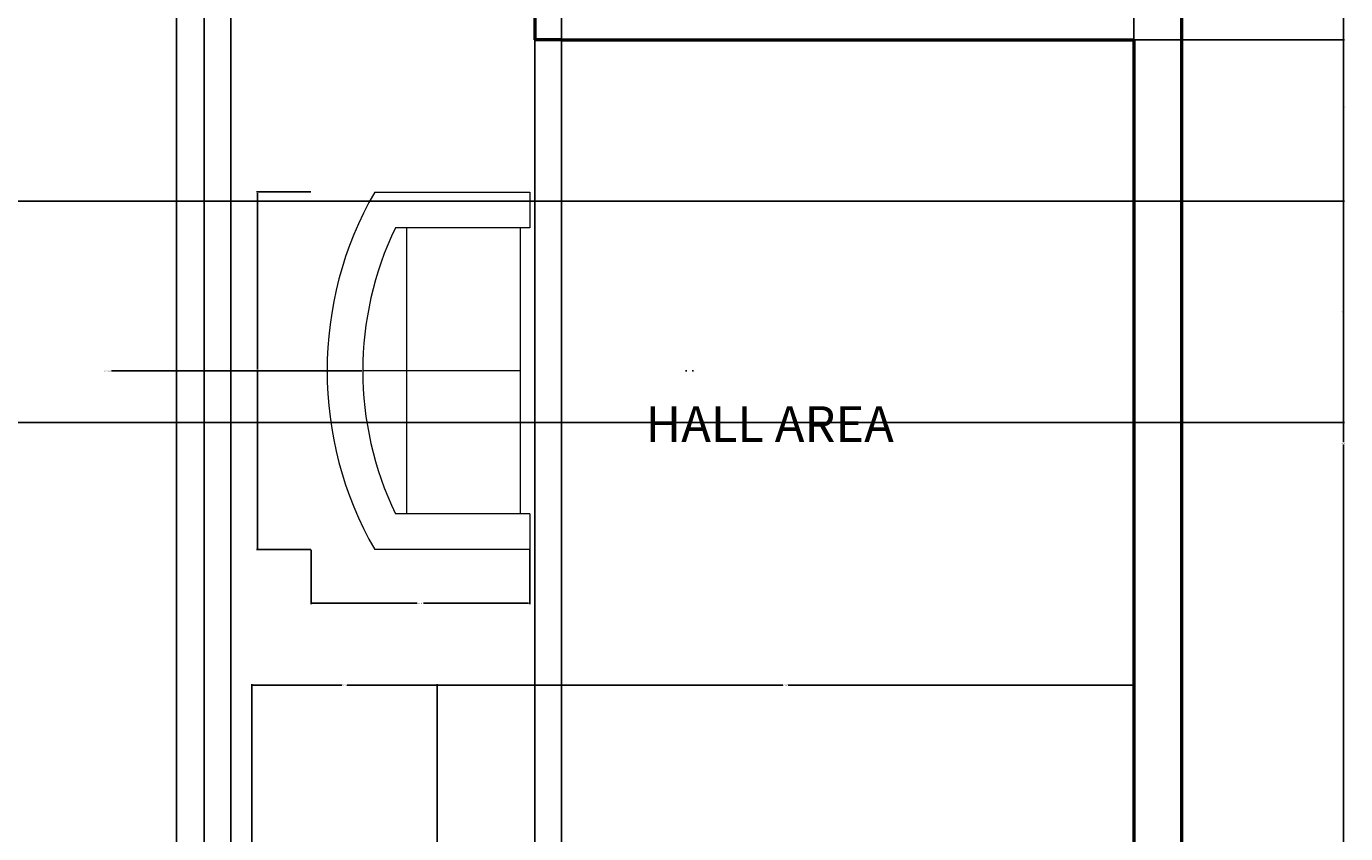
# Model space of a CAD drawing. Units: inches. Extents: x 2907 to 3328, y 1715 to 2286.
# Tile 4 of 5: x 3107 to 3328, y 1969 to 2105. Entities that reach past the tile are written whole.
import ezdxf

# ---------------------------------------------------------------- set-up
doc = ezdxf.new("R2010")
doc.units = ezdxf.units.IN
for name, color, linetype, lineweight in [('A-ANNO-DIMS', 2, 'Continuous', 18), ('A-AREA-IDEN', 7, 'Continuous', 25), ('A-FURN', 8, 'Continuous', 18), ('A-WALL', 7, 'Continuous', 50)]:
    doc.layers.add(name, color=color, linetype=linetype, lineweight=lineweight)
doc.styles.get("Standard").update_dxf_attribs({"font": 'arial.ttf'})
doc.dimstyles.get("Standard").update_dxf_attribs({"dimtxt": 0.18, "dimasz": 0.18, "dimexe": 0.18, "dimexo": 0.0625, "dimgap": 0.09, "dimtad": 0, "dimtih": 1, "dimtoh": 1, "dimdec": 4, "dimzin": 0, "dimdsep": 46, "dimtxsty": 'Standard', "dimcen": 0.09, "dimadec": 0, "dimazin": 0, "dimtfac": 1, "dimtdec": 4, "dimtofl": 0, "dimtmove": 0, "dimatfit": 3, "dimfxl": 1, "dimtolj": 1, "dimtzin": 0, "dimarcsym": 0})

# ---------------------------------------------------------------- blocks, each defined once
blk = doc.blocks.new('Sofa - Roundback Loveseat 5 ft.')
for p, q in [((0, -32.44198), (0, -5.99998)), ((-24, -33.99998), (-24, -11.46958)), ((24.00004, -33.99998), (24.00004, -11.46958)), ((-23.9998, -13.38178), (23.99986, -13.38178)), ((-24, -32.44198), (24.00004, -32.44198))]:
    blk.add_line(p, q)
for points in [[(-24, -33.99998), (-30, -33.99998), (-30, -7.99998)], [(30.00004, -7.99998), (30.00004, -33.99998), (24.00004, -33.99998)]]:
    blk.add_lwpolyline(points)
for centre, radius, start, end in [((0, -60.24998), 60.24998, 60.13715, 119.8628), ((0, -61.38438), 55.38444, 64.32083, 115.6792)]:
    blk.add_arc(centre, radius, start, end)
blk = doc.blocks.new('*D7')
at = {"layer": 'A-ANNO-DIMS', "color": 0, "lineweight": -2, "transparency": 16777216}
for p, q in [((3154.5, 2076.78), (3145.38, 2076.78)), ((3145.56, 2076.6), (3145.56, 2046.96)), ((3145.56, 2016.96), (3145.56, 2046.59)), ((3154.5, 2016.78), (3145.38, 2016.78))]:
    blk.add_line(p, q, dxfattribs=at)
at = {"layer": 'A-ANNO-DIMS', "color": 0, "transparency": 16777216}
for points in [[(3145.53, 2076.6), (3145.59, 2076.6), (3145.56, 2076.78)], [(3145.53, 2016.96), (3145.59, 2016.96), (3145.56, 2016.78)]]:
    blk.add_solid(points, dxfattribs=at)
at = {"layer": 'Defpoints', "color": 0, "transparency": 16777216}
for p in [(3145.56, 2076.78), (3154.56, 2076.78), (3154.56, 2016.78)]:
    blk.add_point(p, dxfattribs=at)
at = {"layer": 'A-ANNO-DIMS', "color": 0, "transparency": 16777216, "insert": (3145.56, 2046.78), "char_height": 0.18, "attachment_point": 5}
blk.add_mtext('\\A1;LOVESEAT 60 TYP.', dxfattribs=at)
blk = doc.blocks.new('*D8')
at = {"layer": 'A-ANNO-DIMS', "color": 0, "lineweight": -2, "transparency": 16777216}
for p, q in [((3154.56, 2016.72), (3154.56, 2007.6)), ((3191.23, 2016.72), (3191.23, 2007.6)), ((3154.74, 2007.78), (3172.37, 2007.78)), ((3191.05, 2007.78), (3173.42, 2007.78))]:
    blk.add_line(p, q, dxfattribs=at)
at = {"layer": 'A-ANNO-DIMS', "color": 0, "transparency": 16777216}
for points in [[(3154.74, 2007.81), (3154.74, 2007.75), (3154.56, 2007.78)], [(3191.05, 2007.81), (3191.05, 2007.75), (3191.23, 2007.78)]]:
    blk.add_solid(points, dxfattribs=at)
at = {"layer": 'Defpoints', "color": 0, "transparency": 16777216}
for p in [(3154.56, 2016.78), (3191.23, 2016.78), (3154.56, 2007.78)]:
    blk.add_point(p, dxfattribs=at)
at = {"layer": 'A-ANNO-DIMS', "color": 0, "transparency": 16777216, "insert": (3172.9, 2007.78), "char_height": 0.18, "attachment_point": 5}
blk.add_mtext('\\A1;37 TYP.', dxfattribs=at)
blk = doc.blocks.new('*D17')
at = {"layer": 'A-ANNO-DIMS', "color": 0, "lineweight": -2, "transparency": 16777216}
for p, q in [((3080.59, 2250.77), (3080.59, 1715.5)), ((3192.09, 2250.77), (3192.09, 1715.5)), ((3080.77, 1715.68), (3135.95, 1715.68)), ((3191.91, 1715.68), (3136.73, 1715.68))]:
    blk.add_line(p, q, dxfattribs=at)
at = {"layer": 'A-ANNO-DIMS', "color": 0, "transparency": 16777216}
for points in [[(3080.77, 1715.71), (3080.77, 1715.65), (3080.59, 1715.68)], [(3191.91, 1715.71), (3191.91, 1715.65), (3192.09, 1715.68)]]:
    blk.add_solid(points, dxfattribs=at)
at = {"layer": 'Defpoints', "color": 0, "transparency": 16777216}
for p in [(3080.59, 2250.83), (3192.09, 2250.83), (3192.09, 1715.68)]:
    blk.add_point(p, dxfattribs=at)
at = {"layer": 'A-ANNO-DIMS', "color": 0, "transparency": 16777216, "insert": (3136.34, 1715.68), "char_height": 0.18, "attachment_point": 5}
blk.add_mtext('\\A1;111.5', dxfattribs=at)
blk = doc.blocks.new('*D18')
at = {"layer": 'A-ANNO-DIMS', "color": 0, "lineweight": -2, "transparency": 16777216}
for p, q in [((3196.59, 2250.77), (3196.59, 1715.5)), ((3292.59, 2250.77), (3292.59, 1715.5)), ((3196.77, 1715.68), (3244.37, 1715.68)), ((3292.41, 1715.68), (3244.81, 1715.68))]:
    blk.add_line(p, q, dxfattribs=at)
at = {"layer": 'A-ANNO-DIMS', "color": 0, "transparency": 16777216}
for points in [[(3196.77, 1715.71), (3196.77, 1715.65), (3196.59, 1715.68)], [(3292.41, 1715.71), (3292.41, 1715.65), (3292.59, 1715.68)]]:
    blk.add_solid(points, dxfattribs=at)
at = {"layer": 'Defpoints', "color": 0, "transparency": 16777216}
for p in [(3196.59, 2250.83), (3292.59, 2250.83), (3292.59, 1715.68)]:
    blk.add_point(p, dxfattribs=at)
at = {"layer": 'A-ANNO-DIMS', "color": 0, "transparency": 16777216, "insert": (3244.59, 1715.68), "char_height": 0.18, "attachment_point": 5}
blk.add_mtext('\\A1;96', dxfattribs=at)
blk = doc.blocks.new('*D29')
at = {"layer": 'A-ANNO-DIMS', "color": 0, "lineweight": -2, "transparency": 16777216}
for p, q in [((3292.65, 2102.33), (3327.92, 2102.33)), ((3327.74, 2102.15), (3327.74, 2034.76)), ((3327.74, 1967.01), (3327.74, 2034.4)), ((3292.65, 1966.83), (3327.92, 1966.83))]:
    blk.add_line(p, q, dxfattribs=at)
at = {"layer": 'A-ANNO-DIMS', "color": 0, "transparency": 16777216}
for points in [[(3327.71, 2102.15), (3327.77, 2102.15), (3327.74, 2102.33)], [(3327.71, 1967.01), (3327.77, 1967.01), (3327.74, 1966.83)]]:
    blk.add_solid(points, dxfattribs=at)
at = {"layer": 'Defpoints', "color": 0, "transparency": 16777216}
for p in [(3292.59, 2102.33), (3327.74, 2102.33), (3292.59, 1966.83)]:
    blk.add_point(p, dxfattribs=at)
at = {"layer": 'A-ANNO-DIMS', "color": 0, "transparency": 16777216, "insert": (3327.74, 2034.58), "char_height": 0.18, "attachment_point": 5}
blk.add_mtext('\\A1;135.5', dxfattribs=at)
blk = doc.blocks.new('*D32')
at = {"layer": 'A-ANNO-DIMS', "color": 0, "lineweight": -2, "transparency": 16777216}
for p, q in [((3141.09, 1786.89), (3141.09, 2286.16)), ((3141.27, 2285.98), (3216.45, 2285.98)), ((3292.41, 2285.98), (3217.23, 2285.98)), ((3292.59, 1786.89), (3292.59, 2286.16))]:
    blk.add_line(p, q, dxfattribs=at)
at = {"layer": 'A-ANNO-DIMS', "color": 0, "transparency": 16777216}
for points in [[(3141.27, 2286.01), (3141.27, 2285.95), (3141.09, 2285.98)], [(3292.41, 2286.01), (3292.41, 2285.95), (3292.59, 2285.98)]]:
    blk.add_solid(points, dxfattribs=at)
at = {"layer": 'Defpoints', "color": 0, "transparency": 16777216}
for p in [(3292.59, 2285.98), (3141.09, 1786.83), (3292.59, 1786.83)]:
    blk.add_point(p, dxfattribs=at)
at = {"layer": 'A-ANNO-DIMS', "color": 0, "transparency": 16777216, "insert": (3216.84, 2285.98), "char_height": 0.18, "attachment_point": 5}
blk.add_mtext('\\A1;151.5', dxfattribs=at)
blk = doc.blocks.new('*D34')
at = {"layer": 'A-ANNO-DIMS', "color": 0, "lineweight": -2, "transparency": 16777216}
for p, q in [((3074.5, 1778.89), (3074.5, 2286.16)), ((3074.68, 2285.98), (3102.84, 2285.98)), ((3131.79, 2285.98), (3103.63, 2285.98)), ((3131.97, 1778.89), (3131.97, 2286.16))]:
    blk.add_line(p, q, dxfattribs=at)
at = {"layer": 'A-ANNO-DIMS', "color": 0, "transparency": 16777216}
for points in [[(3074.68, 2286.01), (3074.68, 2285.95), (3074.5, 2285.98)], [(3131.79, 2286.01), (3131.79, 2285.95), (3131.97, 2285.98)]]:
    blk.add_solid(points, dxfattribs=at)
at = {"layer": 'Defpoints', "color": 0, "transparency": 16777216}
for p in [(3131.97, 2285.98), (3074.5, 1778.83), (3131.97, 1778.83)]:
    blk.add_point(p, dxfattribs=at)
at = {"layer": 'A-ANNO-DIMS', "color": 0, "transparency": 16777216, "insert": (3103.24, 2285.98), "char_height": 0.18, "attachment_point": 5}
blk.add_mtext('\\A1;57.47', dxfattribs=at)
blk = doc.blocks.new('*D38')
at = {"layer": 'A-ANNO-DIMS', "color": 0, "lineweight": -2, "transparency": 16777216}
for p, q in [((3080.65, 2075.23), (3327.92, 2075.23)), ((3327.74, 2075.05), (3327.74, 2056.85)), ((3327.74, 2038.29), (3327.74, 2056.48)), ((3080.65, 2038.11), (3327.92, 2038.11))]:
    blk.add_line(p, q, dxfattribs=at)
at = {"layer": 'A-ANNO-DIMS', "color": 0, "transparency": 16777216}
for points in [[(3327.71, 2075.05), (3327.77, 2075.05), (3327.74, 2075.23)], [(3327.71, 2038.29), (3327.77, 2038.29), (3327.74, 2038.11)]]:
    blk.add_solid(points, dxfattribs=at)
at = {"layer": 'Defpoints', "color": 0, "transparency": 16777216}
for p in [(3080.59, 2075.23), (3327.74, 2075.23), (3080.59, 2038.11)]:
    blk.add_point(p, dxfattribs=at)
at = {"layer": 'A-ANNO-DIMS', "color": 0, "transparency": 16777216, "insert": (3327.74, 2056.67), "char_height": 0.18, "attachment_point": 5}
blk.add_mtext('\\A1;37.12', dxfattribs=at)
blk = doc.blocks.new('*D39')
at = {"layer": 'A-ANNO-DIMS', "color": 0, "lineweight": -2, "transparency": 16777216}
for p, q in [((3076.15, 2106.83), (3327.92, 2106.83)), ((3327.74, 2106.65), (3327.74, 2091.21)), ((3327.74, 2075.41), (3327.74, 2090.85)), ((3080.65, 2075.23), (3327.92, 2075.23))]:
    blk.add_line(p, q, dxfattribs=at)
at = {"layer": 'A-ANNO-DIMS', "color": 0, "transparency": 16777216}
for points in [[(3327.71, 2106.65), (3327.77, 2106.65), (3327.74, 2106.83)], [(3327.71, 2075.41), (3327.77, 2075.41), (3327.74, 2075.23)]]:
    blk.add_solid(points, dxfattribs=at)
at = {"layer": 'Defpoints', "color": 0, "transparency": 16777216}
for p in [(3076.09, 2106.83), (3327.74, 2106.83), (3080.59, 2075.23)]:
    blk.add_point(p, dxfattribs=at)
at = {"layer": 'A-ANNO-DIMS', "color": 0, "transparency": 16777216, "insert": (3327.74, 2091.03), "char_height": 0.18, "attachment_point": 5}
blk.add_mtext('\\A1;31.604', dxfattribs=at)
blk = doc.blocks.new('*D42')
at = {"layer": 'A-ANNO-DIMS', "color": 0, "lineweight": -2, "transparency": 16777216}
for p, q in [((3144.59, 1966.89), (3144.59, 1994.16)), ((3175.72, 1966.89), (3175.72, 1994.16)), ((3144.77, 1993.98), (3159.69, 1993.98)), ((3175.54, 1993.98), (3160.62, 1993.98))]:
    blk.add_line(p, q, dxfattribs=at)
at = {"layer": 'A-ANNO-DIMS', "color": 0, "transparency": 16777216}
for points in [[(3144.77, 1994.01), (3144.77, 1993.95), (3144.59, 1993.98)], [(3175.54, 1994.01), (3175.54, 1993.95), (3175.72, 1993.98)]]:
    blk.add_solid(points, dxfattribs=at)
at = {"layer": 'Defpoints', "color": 0, "transparency": 16777216}
for p in [(3175.72, 1993.98), (3144.59, 1966.83), (3175.72, 1966.83)]:
    blk.add_point(p, dxfattribs=at)
at = {"layer": 'A-ANNO-DIMS', "color": 0, "transparency": 16777216, "insert": (3160.16, 1993.98), "char_height": 0.18, "attachment_point": 5}
blk.add_mtext('\\A1;31.134', dxfattribs=at)
blk = doc.blocks.new('*D43')
at = {"layer": 'A-ANNO-DIMS', "color": 0, "lineweight": -2, "transparency": 16777216}
for p, q in [((3175.72, 1966.89), (3175.72, 1994.16)), ((3292.59, 1966.89), (3292.59, 1994.16)), ((3175.9, 1993.98), (3233.7, 1993.98)), ((3292.41, 1993.98), (3234.61, 1993.98))]:
    blk.add_line(p, q, dxfattribs=at)
at = {"layer": 'A-ANNO-DIMS', "color": 0, "transparency": 16777216}
for points in [[(3175.9, 1994.01), (3175.9, 1993.95), (3175.72, 1993.98)], [(3292.41, 1994.01), (3292.41, 1993.95), (3292.59, 1993.98)]]:
    blk.add_solid(points, dxfattribs=at)
at = {"layer": 'Defpoints', "color": 0, "transparency": 16777216}
for p in [(3292.59, 1993.98), (3175.72, 1966.83), (3292.59, 1966.83)]:
    blk.add_point(p, dxfattribs=at)
at = {"layer": 'A-ANNO-DIMS', "color": 0, "transparency": 16777216, "insert": (3234.16, 1993.98), "char_height": 0.18, "attachment_point": 5}
blk.add_mtext('\\A1;116.87', dxfattribs=at)
blk = doc.blocks.new('*D56')
at = {"layer": 'A-ANNO-DIMS', "color": 0, "lineweight": -2, "transparency": 16777216}
for p, q in [((2942.59, 1786.89), (2942.59, 2286.16)), ((2942.77, 2285.98), (3039.31, 2285.98)), ((3136.41, 2285.98), (3039.87, 2285.98)), ((3136.59, 1786.89), (3136.59, 2286.16))]:
    blk.add_line(p, q, dxfattribs=at)
at = {"layer": 'A-ANNO-DIMS', "color": 0, "transparency": 16777216}
for points in [[(2942.77, 2286.01), (2942.77, 2285.95), (2942.59, 2285.98)], [(3136.41, 2286.01), (3136.41, 2285.95), (3136.59, 2285.98)]]:
    blk.add_solid(points, dxfattribs=at)
at = {"layer": 'Defpoints', "color": 0, "transparency": 16777216}
for p in [(3136.59, 2285.98), (2942.59, 1786.83), (3136.59, 1786.83)]:
    blk.add_point(p, dxfattribs=at)
at = {"layer": 'A-ANNO-DIMS', "color": 0, "transparency": 16777216, "insert": (3039.59, 2285.98), "char_height": 0.18, "attachment_point": 5}
blk.add_mtext('\\A1;194', dxfattribs=at)
blk = doc.blocks.new('*D61')
at = {"layer": 'A-ANNO-DIMS', "color": 0, "lineweight": -2, "transparency": 16777216}
for p, q in [((3121.08, 2046.78), (3157.05, 2046.78)), ((3217.39, 2046.78), (3217.57, 2046.78)), ((3217.48, 2046.69), (3217.48, 2046.87))]:
    blk.add_line(p, q, dxfattribs=at)
at = {"layer": 'A-ANNO-DIMS', "color": 0, "transparency": 16777216}
blk.add_solid([(3157.05, 2046.81), (3157.05, 2046.75), (3157.23, 2046.78)], dxfattribs=at)
at = {"layer": 'Defpoints', "color": 0, "transparency": 16777216}
for p in [(3157.23, 2046.78), (3217.48, 2046.78)]:
    blk.add_point(p, dxfattribs=at)
at = {"layer": 'A-ANNO-DIMS', "color": 0, "transparency": 16777216, "insert": (3120.4, 2046.78), "char_height": 0.18, "attachment_point": 5}
blk.add_mtext('\\A1;2X R60.25', dxfattribs=at)
blk = doc.blocks.new('*D62')
at = {"layer": 'A-ANNO-DIMS', "color": 0, "lineweight": -2, "transparency": 16777216}
for p, q in [((3130, 2046.78), (3163.05, 2046.78)), ((3218.52, 2046.78), (3218.7, 2046.78)), ((3218.61, 2046.69), (3218.61, 2046.87))]:
    blk.add_line(p, q, dxfattribs=at)
at = {"layer": 'A-ANNO-DIMS', "color": 0, "transparency": 16777216}
blk.add_solid([(3163.05, 2046.81), (3163.05, 2046.75), (3163.23, 2046.78)], dxfattribs=at)
at = {"layer": 'Defpoints', "color": 0, "transparency": 16777216}
for p in [(3163.23, 2046.78), (3218.61, 2046.78)]:
    blk.add_point(p, dxfattribs=at)
at = {"layer": 'A-ANNO-DIMS', "color": 0, "transparency": 16777216, "insert": (3129.32, 2046.78), "char_height": 0.18, "attachment_point": 5}
blk.add_mtext('\\A1;2X R55.38', dxfattribs=at)

msp = doc.modelspace()

# ---------------------------------------------------------------- linework, layer by layer
at = {"layer": 'A-WALL'}
for p, q in [((3300.5892, 2258.8301), (3300.5892, 1778.8301)), ((3192.0892, 2106.8301), (3192.0892, 2102.3301)), ((3196.5892, 2102.3301), (3192.0892, 2102.3301)), ((3196.5892, 2102.3301), (3292.5892, 2102.3301)), ((3292.5892, 2102.3301), (3292.5892, 1966.8301))]:
    msp.add_line(p, q, dxfattribs=at)

# ---------------------------------------------------------------- block references
at = {"layer": 'A-FURN', "rotation": 90}
msp.add_blockref('Sofa - Roundback Loveseat 5 ft.', (3157.2292, 2046.7778), dxfattribs=at)

# ---------------------------------------------------------------- texts
at = {"layer": 'A-AREA-IDEN', "insert": (3210.6903, 2040.8254), "char_height": 6, "attachment_point": 1}
msp.add_mtext_dynamic_manual_height_columns('HALL AREA ', width=50.965346, gutter_width=12.5, heights=[0], dxfattribs=at)

# ---------------------------------------------------------------- dimensions: what is measured, and where the dimension line sits
at = {"layer": 'A-ANNO-DIMS'}
for base, p1, p2, override, picture, middle in [((3136.5892, 2285.9816), (2942.5892, 1786.8301), (3136.5892, 1786.8301), {"dimdec": 0, "dimlfac": 1, "dimrnd": 0, "dimzin": 0, "dimdsep": 46, "dimlunit": 2}, '*D56', (3039.5892, 2285.9816)), ((3131.9734, 2285.9816), (3074.499, 1778.8301), (3131.9734, 1778.8301), {"dimdec": 2, "dimlfac": 1, "dimrnd": 0, "dimzin": 0, "dimdsep": 46, "dimlunit": 2}, '*D34', (3103.2362, 2285.9816)), ((3292.5892, 2285.9816), (3141.0892, 1786.8301), (3292.5892, 1786.8301), {"dimdec": 1, "dimlfac": 1, "dimrnd": 0, "dimzin": 0, "dimdsep": 46, "dimlunit": 2}, '*D32', (3216.8392, 2285.9816)), ((3192.0892, 1715.6786), (3080.5892, 2250.8301), (3192.0892, 2250.8301), {"dimdec": 1, "dimlfac": 1, "dimrnd": 0, "dimzin": 0, "dimdsep": 46, "dimlunit": 2}, '*D17', (3136.3392, 1715.6786)), ((3292.5892, 1715.6786), (3196.5892, 2250.8301), (3292.5892, 2250.8301), {"dimdec": 0, "dimlfac": 1, "dimrnd": 0, "dimzin": 0, "dimdsep": 46, "dimlunit": 2}, '*D18', (3244.5892, 1715.6786)), ((3175.7234, 1993.9816), (3144.5892, 1966.8301), (3175.7234, 1966.8301), {"dimdec": 3, "dimlfac": 1, "dimrnd": 0, "dimzin": 0, "dimdsep": 46, "dimlunit": 2}, '*D42', (3160.1563, 1993.9816))]:
    dim = msp.add_linear_dim(base=base, p1=p1, p2=p2, dimstyle='Standard', override=override, dxfattribs=at)
    dim.commit()
    dim.dimension.update_dxf_attribs({"geometry": picture, "text_midpoint": middle})
for base, p1, p2, angle, override, picture, middle in [((3327.7407, 2106.8301), (3080.5892, 2075.2259), (3076.0892, 2106.8301), 90, {"dimdec": 3, "dimlfac": 1, "dimrnd": 0, "dimzin": 0, "dimdsep": 46, "dimlunit": 2}, '*D39', (3327.7407, 2091.028)), ((3327.7407, 2102.3301), (3292.5892, 1966.8301), (3292.5892, 2102.3301), 90, {"dimdec": 1, "dimlfac": 1, "dimrnd": 0, "dimzin": 0, "dimdsep": 46, "dimlunit": 2}, '*D29', (3327.7407, 2034.5801)), ((3327.7407, 2075.2259), (3080.5892, 2038.1078), (3080.5892, 2075.2259), 90, {"dimdec": 2, "dimlfac": 1, "dimrnd": 0, "dimzin": 0, "dimdsep": 46, "dimlunit": 2}, '*D38', (3327.7407, 2056.6669)), ((3292.5892, 1993.9816), (3175.7234, 1966.8301), (3292.5892, 1966.8301), 0, {"dimdec": 2, "dimlfac": 1, "dimrnd": 0, "dimzin": 0, "dimdsep": 46, "dimlunit": 2}, '*D43', (3234.1563, 1993.9816))]:
    dim = msp.add_linear_dim(base=base, p1=p1, p2=p2, angle=angle, dimstyle='Standard', override=override, dxfattribs=at)
    dim.commit()
    dim.dimension.update_dxf_attribs({"geometry": picture, "text_midpoint": middle})
for base, p1, p2, angle, text, picture, middle in [((3145.5625, 2076.7779), (3154.5625, 2016.7778), (3154.5625, 2076.7779), 90, 'LOVESEAT <> TYP.', '*D7', (3145.5625, 2046.7778)), ((3154.5625, 2007.7778), (3191.2291, 2016.7778), (3154.5625, 2016.7778), 180, '<> TYP.', '*D8', (3172.8958, 2007.7778))]:
    dim = msp.add_linear_dim(base=base, p1=p1, p2=p2, angle=angle, text=text, dimstyle='Standard', override={"dimdec": 0, "dimlfac": 1, "dimrnd": 0, "dimzin": 0, "dimdsep": 46, "dimlunit": 2}, dxfattribs=at)
    dim.commit()
    dim.dimension.update_dxf_attribs({"geometry": picture, "text_midpoint": middle})
for center, mpoint, picture, middle in [((3217.4791, 2046.7778), (3157.2292, 2046.778), '*D61', (3121.0792, 2046.7781)), ((3218.6135, 2046.7778), (3163.2291, 2046.778), '*D62', (3129.9984, 2046.7781))]:
    dim = msp.add_radius_dim(center=center, mpoint=mpoint, text='2X <>', dimstyle='Standard', override={"dimdec": 2, "dimlfac": 1, "dimrnd": 0, "dimzin": 0, "dimdsep": 46, "dimlunit": 2}, dxfattribs=at)
    dim.commit()
    dim.dimension.update_dxf_attribs({"geometry": picture, "text_midpoint": middle, "dimtype": 164})

doc.saveas('drawing.dxf')
